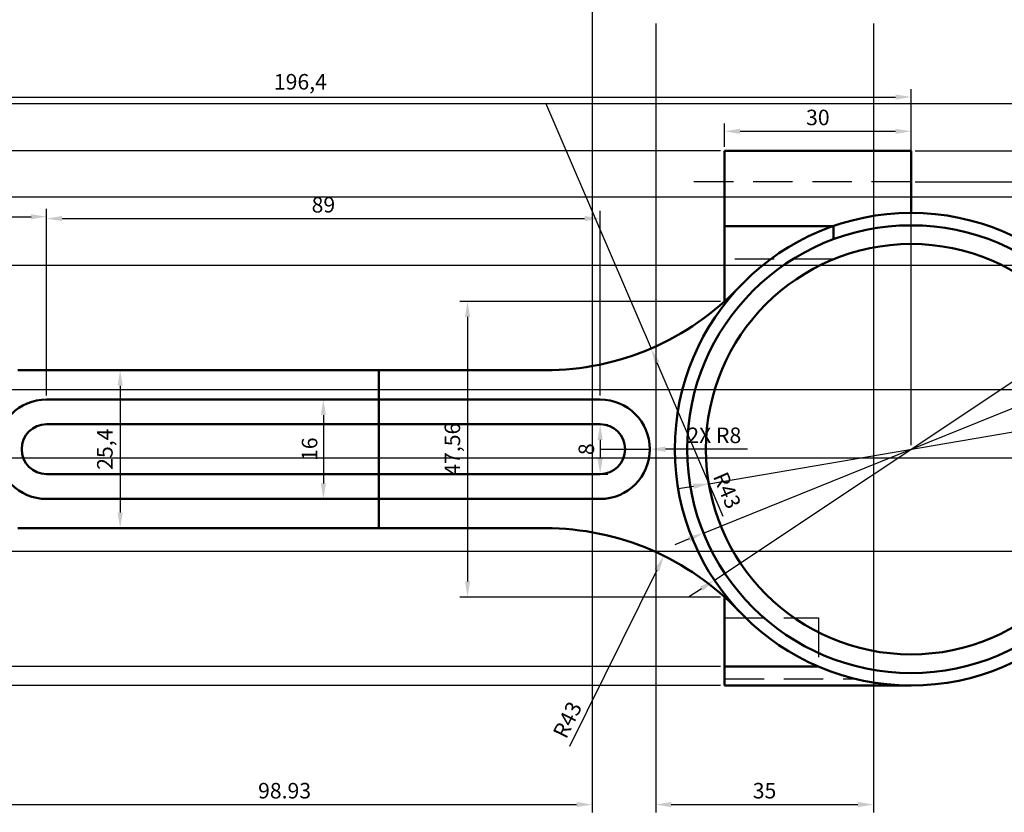
# Model space of a CAD drawing. Units: millimetres. Extents: x 1594 to 1992, y 1694 to 1927.
# Tile 2 of 4: x 1698 to 1856, y 1694 to 1822. Entities that reach past the tile are written whole.
import ezdxf

# ---------------------------------------------------------------- set-up
doc = ezdxf.new("R2010")
doc.units = ezdxf.units.MM
doc.linetypes.add('HIDDEN', pattern=[9.525, 6.35, -3.175])
for name, color, linetype, lineweight in [('M-DIMS', 2, 'Continuous', 25), ('M-HIDN', 4, 'HIDDEN', 25), ('M-OUTL', 7, 'Continuous', 50)]:
    doc.layers.add(name, color=color, linetype=linetype, lineweight=lineweight)
doc.styles.get("Standard").update_dxf_attribs({"font": 'arial.ttf'})
doc.dimstyles.new('ISO-25', dxfattribs={"dimtxt": 2.5, "dimasz": 2.5, "dimexe": 1.25, "dimexo": 0.625, "dimtad": 1, "dimtxsty": 'Standard', "dimcen": 2.5, "dimadec": 0, "dimazin": 0, "dimtfac": 1, "dimtmove": 0, "dimatfit": 3, "dimfxl": 1, "dimarcsym": 0})

# ---------------------------------------------------------------- blocks, each defined once
blk = doc.blocks.new('*D13')
at = {"layer": 'Defpoints', "color": 0, "transparency": 16777216}
for p in [(1701.91, 1789.89), (1701.91, 1760.5), (1669.71, 1752.5)]:
    blk.add_point(p, dxfattribs=at)
at = {"layer": 'M-DIMS', "color": 0, "lineweight": -2, "transparency": 16777216}
for p, q in [((1669.71, 1753.13), (1669.71, 1791.14)), ((1701.91, 1761.13), (1701.91, 1791.14)), ((1672.21, 1789.89), (1699.41, 1789.89))]:
    blk.add_line(p, q, dxfattribs=at)
at = {"layer": 'M-DIMS', "color": 0, "transparency": 16777216}
for points in [[(1672.21, 1790.3), (1672.21, 1789.47), (1669.71, 1789.89)], [(1699.41, 1790.3), (1699.41, 1789.47), (1701.91, 1789.89)]]:
    blk.add_solid(points, dxfattribs=at)
at = {"layer": 'M-DIMS', "color": 0, "transparency": 16777216, "insert": (1685.81, 1792.01), "char_height": 2.5, "attachment_point": 5}
blk.add_mtext('32,2', dxfattribs=at)
blk = doc.blocks.new('*D14')
at = {"layer": 'Defpoints', "color": 0, "transparency": 16777216}
for p in [(1790.91, 1789.59), (1701.91, 1760.5), (1790.91, 1760.5)]:
    blk.add_point(p, dxfattribs=at)
at = {"layer": 'M-DIMS', "color": 0, "lineweight": -2, "transparency": 16777216}
for p, q in [((1701.91, 1761.13), (1701.91, 1790.84)), ((1790.91, 1761.13), (1790.91, 1790.84)), ((1704.41, 1789.59), (1788.41, 1789.59))]:
    blk.add_line(p, q, dxfattribs=at)
at = {"layer": 'M-DIMS', "color": 0, "transparency": 16777216}
for points in [[(1704.41, 1790.01), (1704.41, 1789.18), (1701.91, 1789.59)], [(1788.41, 1790.01), (1788.41, 1789.18), (1790.91, 1789.59)]]:
    blk.add_solid(points, dxfattribs=at)
at = {"layer": 'M-DIMS', "color": 0, "transparency": 16777216, "insert": (1746.41, 1791.49), "char_height": 2.5, "attachment_point": 5}
blk.add_mtext('89', dxfattribs=at)
blk = doc.blocks.new('*D16')
at = {"layer": 'Defpoints', "color": 0, "transparency": 16777216}
for p in [(1840.91, 1809.14), (1644.51, 1752.5), (1840.91, 1752.5)]:
    blk.add_point(p, dxfattribs=at)
at = {"layer": 'M-DIMS', "color": 0, "lineweight": -2, "transparency": 16777216}
for p, q in [((1644.51, 1753.13), (1644.51, 1810.39)), ((1840.91, 1753.13), (1840.91, 1810.39)), ((1647.01, 1809.14), (1838.41, 1809.14))]:
    blk.add_line(p, q, dxfattribs=at)
at = {"layer": 'M-DIMS', "color": 0, "transparency": 16777216}
for points in [[(1647.01, 1809.56), (1647.01, 1808.72), (1644.51, 1809.14)], [(1838.41, 1809.56), (1838.41, 1808.72), (1840.91, 1809.14)]]:
    blk.add_solid(points, dxfattribs=at)
at = {"layer": 'M-DIMS', "color": 0, "transparency": 16777216, "insert": (1742.71, 1811.27), "char_height": 2.5, "attachment_point": 5}
blk.add_mtext('196,4', dxfattribs=at)
blk = doc.blocks.new('*D17')
at = {"layer": 'Defpoints', "color": 0, "transparency": 16777216}
for p in [(1840.91, 1803.63), (1810.91, 1800.5), (1840.91, 1800.5)]:
    blk.add_point(p, dxfattribs=at)
at = {"layer": 'M-DIMS', "color": 0, "lineweight": -2, "transparency": 16777216}
for p, q in [((1810.91, 1801.13), (1810.91, 1804.88)), ((1840.91, 1801.13), (1840.91, 1804.88)), ((1813.41, 1803.63), (1838.41, 1803.63))]:
    blk.add_line(p, q, dxfattribs=at)
at = {"layer": 'M-DIMS', "color": 0, "transparency": 16777216}
for points in [[(1813.41, 1804.04), (1813.41, 1803.21), (1810.91, 1803.63)], [(1838.41, 1804.04), (1838.41, 1803.21), (1840.91, 1803.63)]]:
    blk.add_solid(points, dxfattribs=at)
at = {"layer": 'M-DIMS', "color": 0, "transparency": 16777216, "insert": (1825.91, 1805.53), "char_height": 2.5, "attachment_point": 5}
blk.add_mtext('30', dxfattribs=at)
blk = doc.blocks.new('*D18')
at = {"layer": 'Defpoints', "color": 0, "transparency": 16777216}
for p in [(1726.28, 1765.2), (1713.73, 1739.8), (1726.28, 1739.8)]:
    blk.add_point(p, dxfattribs=at)
at = {"layer": 'M-DIMS', "color": 0, "lineweight": -2, "transparency": 16777216}
for p, q in [((1725.66, 1765.2), (1712.48, 1765.2)), ((1713.73, 1762.7), (1713.73, 1742.3)), ((1725.66, 1739.8), (1712.48, 1739.8))]:
    blk.add_line(p, q, dxfattribs=at)
at = {"layer": 'M-DIMS', "color": 0, "transparency": 16777216}
for points in [[(1713.32, 1762.7), (1714.15, 1762.7), (1713.73, 1765.2)], [(1713.32, 1742.3), (1714.15, 1742.3), (1713.73, 1739.8)]]:
    blk.add_solid(points, dxfattribs=at)
at = {"layer": 'M-DIMS', "color": 0, "transparency": 16777216, "insert": (1711.6, 1752.5), "char_height": 2.5, "attachment_point": 5, "rotation": 90}
blk.add_mtext('25,4', dxfattribs=at)
blk = doc.blocks.new('*D19')
at = {"layer": 'Defpoints', "color": 0, "transparency": 16777216}
for p in [(1746.41, 1760.5), (1746.41, 1744.5), (1746.41, 1744.5)]:
    blk.add_point(p, dxfattribs=at)
at = {"layer": 'M-DIMS', "color": 0, "lineweight": -2, "transparency": 16777216}
for p, q in [((1747.03, 1760.5), (1747.66, 1760.5)), ((1746.41, 1758), (1746.41, 1747)), ((1747.03, 1744.5), (1747.66, 1744.5))]:
    blk.add_line(p, q, dxfattribs=at)
at = {"layer": 'M-DIMS', "color": 0, "transparency": 16777216}
for points in [[(1745.99, 1758), (1746.82, 1758), (1746.41, 1760.5)], [(1745.99, 1747), (1746.82, 1747), (1746.41, 1744.5)]]:
    blk.add_solid(points, dxfattribs=at)
at = {"layer": 'M-DIMS', "color": 0, "transparency": 16777216, "insert": (1744.51, 1752.5), "char_height": 2.5, "attachment_point": 5, "rotation": 90}
blk.add_mtext('16', dxfattribs=at)
blk = doc.blocks.new('*D20')
at = {"layer": 'Defpoints', "color": 0, "transparency": 16777216}
for p in [(1746.41, 1756.5), (1746.41, 1748.5), (1790.91, 1748.5)]:
    blk.add_point(p, dxfattribs=at)
at = {"layer": 'M-DIMS', "color": 0, "lineweight": -2, "transparency": 16777216}
for p, q in [((1747.03, 1756.5), (1792.16, 1756.5)), ((1790.91, 1754), (1790.91, 1751)), ((1747.03, 1748.5), (1792.16, 1748.5))]:
    blk.add_line(p, q, dxfattribs=at)
at = {"layer": 'M-DIMS', "color": 0, "transparency": 16777216}
for points in [[(1790.49, 1754), (1791.32, 1754), (1790.91, 1756.5)], [(1790.49, 1751), (1791.32, 1751), (1790.91, 1748.5)]]:
    blk.add_solid(points, dxfattribs=at)
at = {"layer": 'M-DIMS', "color": 0, "transparency": 16777216, "insert": (1789.01, 1752.5), "char_height": 2.5, "attachment_point": 5, "rotation": 90}
blk.add_mtext('8', dxfattribs=at)
blk = doc.blocks.new('*D21')
at = {"layer": 'Defpoints', "color": 0, "transparency": 16777216}
for p in [(1810.91, 1776.28), (1769.59, 1728.73), (1810.91, 1728.73)]:
    blk.add_point(p, dxfattribs=at)
at = {"layer": 'M-DIMS', "color": 0, "lineweight": -2, "transparency": 16777216}
for p, q in [((1810.28, 1776.28), (1768.34, 1776.28)), ((1769.59, 1773.78), (1769.59, 1731.23)), ((1810.28, 1728.73), (1768.34, 1728.73))]:
    blk.add_line(p, q, dxfattribs=at)
at = {"layer": 'M-DIMS', "color": 0, "transparency": 16777216}
for points in [[(1769.18, 1773.78), (1770.01, 1773.78), (1769.59, 1776.28)], [(1769.18, 1731.23), (1770.01, 1731.23), (1769.59, 1728.73)]]:
    blk.add_solid(points, dxfattribs=at)
at = {"layer": 'M-DIMS', "color": 0, "transparency": 16777216, "insert": (1767.47, 1752.5), "char_height": 2.5, "attachment_point": 5, "rotation": 90}
blk.add_mtext('47,56', dxfattribs=at)
blk = doc.blocks.new('*D24')
at = {"layer": 'Defpoints', "color": 0, "transparency": 16777216}
for p in [(1801.16, 1735.35), (1782.1, 1696.8)]:
    blk.add_point(p, dxfattribs=at)
at = {"layer": 'M-DIMS', "color": 0, "lineweight": -2, "transparency": 16777216}
blk.add_line((1786.03, 1704.76), (1800.05, 1733.11), dxfattribs=at)
at = {"layer": 'M-DIMS', "color": 0, "transparency": 16777216}
blk.add_solid([(1799.68, 1733.29), (1800.42, 1732.92), (1801.16, 1735.35)], dxfattribs=at)
at = {"layer": 'M-DIMS', "color": 0, "transparency": 16777216, "insert": (1785.93, 1708.84), "char_height": 2.5, "attachment_point": 5, "rotation": 63.6879}
blk.add_mtext('R43', dxfattribs=at)
blk = doc.blocks.new('*D28')
at = {"layer": 'Defpoints', "color": 0, "transparency": 16777216}
for p in [(1872.54, 1773.56), (1809.27, 1731.45)]:
    blk.add_point(p, dxfattribs=at)
at = {"layer": 'M-DIMS', "color": 0, "lineweight": -2, "transparency": 16777216}
for p, q in [((1891.75, 1786.34), (1874.62, 1774.94)), ((1809.27, 1731.45), (1872.54, 1773.56)), ((1807.19, 1730.07), (1805.11, 1728.68))]:
    blk.add_line(p, q, dxfattribs=at)
at = {"layer": 'M-DIMS', "color": 0, "transparency": 16777216}
for points in [[(1874.39, 1775.29), (1874.85, 1774.59), (1872.54, 1773.56)], [(1806.96, 1730.42), (1807.42, 1729.72), (1809.27, 1731.45)]]:
    blk.add_solid(points, dxfattribs=at)
at = {"layer": 'M-DIMS', "color": 0, "transparency": 16777216, "insert": (1887.51, 1785.89), "char_height": 2.5, "attachment_point": 5, "rotation": 33.6408}
blk.add_mtext('∅76', dxfattribs=at)
blk = doc.blocks.new('*D29')
at = {"layer": 'Defpoints', "color": 0, "transparency": 16777216}
for p in [(1874.28, 1766), (1807.53, 1739.01)]:
    blk.add_point(p, dxfattribs=at)
at = {"layer": 'M-DIMS', "color": 0, "lineweight": -2, "transparency": 16777216}
for p, q in [((1897.51, 1775.4), (1876.6, 1766.94)), ((1807.53, 1739.01), (1874.28, 1766)), ((1805.22, 1738.07), (1802.9, 1737.13))]:
    blk.add_line(p, q, dxfattribs=at)
at = {"layer": 'M-DIMS', "color": 0, "transparency": 16777216}
for points in [[(1876.44, 1767.33), (1876.75, 1766.55), (1874.28, 1766)], [(1805.06, 1738.46), (1805.37, 1737.68), (1807.53, 1739.01)]]:
    blk.add_solid(points, dxfattribs=at)
at = {"layer": 'M-DIMS', "color": 0, "transparency": 16777216, "insert": (1893.28, 1775.81), "char_height": 2.5, "attachment_point": 5, "rotation": 22.0218}
blk.add_mtext('∅72', dxfattribs=at)
blk = doc.blocks.new('*D30')
at = {"layer": 'Defpoints', "color": 0, "transparency": 16777216}
for p in [(1873.44, 1758.06), (1808.38, 1746.95)]:
    blk.add_point(p, dxfattribs=at)
at = {"layer": 'M-DIMS', "color": 0, "lineweight": -2, "transparency": 16777216}
for p, q in [((1899.42, 1762.5), (1875.9, 1758.48)), ((1808.38, 1746.95), (1873.44, 1758.06)), ((1805.91, 1746.53), (1803.45, 1746.11))]:
    blk.add_line(p, q, dxfattribs=at)
at = {"layer": 'M-DIMS', "color": 0, "transparency": 16777216}
for points in [[(1875.83, 1758.89), (1875.97, 1758.07), (1873.44, 1758.06)], [(1805.84, 1746.94), (1805.98, 1746.12), (1808.38, 1746.95)]]:
    blk.add_solid(points, dxfattribs=at)
at = {"layer": 'M-DIMS', "color": 0, "transparency": 16777216, "insert": (1895.37, 1763.81), "char_height": 2.5, "attachment_point": 5, "rotation": 9.6936}
blk.add_mtext('∅66', dxfattribs=at)
blk = doc.blocks.new('*D39')
at = {"layer": 'Defpoints', "color": 0, "transparency": 16777216}
for p in [(1840.91, 1800.5), (1840.91, 1795.5), (1985.18, 1795.5)]:
    blk.add_point(p, dxfattribs=at)
at = {"layer": 'M-DIMS', "color": 0, "lineweight": -2, "transparency": 16777216}
for p, q in [((1985.18, 1803), (1985.18, 1805.5)), ((1841.53, 1800.5), (1986.43, 1800.5)), ((1985.18, 1800.5), (1985.18, 1795.5)), ((1841.53, 1795.5), (1986.43, 1795.5)), ((1985.18, 1793), (1985.18, 1790.5))]:
    blk.add_line(p, q, dxfattribs=at)
at = {"layer": 'M-DIMS', "color": 0, "transparency": 16777216}
for points in [[(1984.76, 1803), (1985.6, 1803), (1985.18, 1800.5)], [(1984.76, 1793), (1985.6, 1793), (1985.18, 1795.5)]]:
    blk.add_solid(points, dxfattribs=at)
at = {"layer": 'M-DIMS', "color": 0, "transparency": 16777216, "insert": (1983.28, 1798), "char_height": 2.5, "attachment_point": 5, "rotation": 90}
blk.add_mtext('5', dxfattribs=at)
blk = doc.blocks.new('*D40')
at = {"layer": 'Defpoints', "color": 0, "transparency": 16777216}
for p in [(1810.91, 1800.5), (1597.57, 1714.5), (1810.91, 1714.5)]:
    blk.add_point(p, dxfattribs=at)
at = {"layer": 'M-DIMS', "color": 0, "lineweight": -2, "transparency": 16777216}
for p, q in [((1810.28, 1800.5), (1596.32, 1800.5)), ((1597.57, 1798), (1597.57, 1717)), ((1810.28, 1714.5), (1596.32, 1714.5))]:
    blk.add_line(p, q, dxfattribs=at)
at = {"layer": 'M-DIMS', "color": 0, "transparency": 16777216}
for points in [[(1597.15, 1798), (1597.99, 1798), (1597.57, 1800.5)], [(1597.15, 1717), (1597.99, 1717), (1597.57, 1714.5)]]:
    blk.add_solid(points, dxfattribs=at)
at = {"layer": 'M-DIMS', "color": 0, "transparency": 16777216, "insert": (1595.67, 1757.5), "char_height": 2.5, "attachment_point": 5, "rotation": 90}
blk.add_mtext('86', dxfattribs=at)
blk = doc.blocks.new('*D41')
at = {"layer": 'Defpoints', "color": 0, "transparency": 16777216}
for p in [(1810.91, 1717.55), (1597.57, 1714.5), (1810.91, 1714.5)]:
    blk.add_point(p, dxfattribs=at)
at = {"layer": 'M-DIMS', "color": 0, "lineweight": -2, "transparency": 16777216}
for p, q in [((1597.57, 1720.05), (1597.57, 1722.55)), ((1810.28, 1717.55), (1596.32, 1717.55)), ((1597.57, 1717.55), (1597.57, 1714.5)), ((1810.28, 1714.5), (1596.32, 1714.5)), ((1597.57, 1712), (1597.57, 1701.74))]:
    blk.add_line(p, q, dxfattribs=at)
at = {"layer": 'M-DIMS', "color": 0, "transparency": 16777216}
for points in [[(1597.15, 1720.05), (1597.99, 1720.05), (1597.57, 1717.55)], [(1597.15, 1712), (1597.99, 1712), (1597.57, 1714.5)]]:
    blk.add_solid(points, dxfattribs=at)
at = {"layer": 'M-DIMS', "color": 0, "transparency": 16777216, "insert": (1595.67, 1705.62), "char_height": 2.5, "attachment_point": 5, "rotation": 90}
blk.add_mtext('3.05', dxfattribs=at)
blk = doc.blocks.new('*D44')
at = {"layer": 'Defpoints', "color": 0, "transparency": 16777216}
for p in [(1932.03, 1782.06), (1597.57, 1762.06), (1932.03, 1762.06)]:
    blk.add_point(p, dxfattribs=at)
at = {"layer": 'M-DIMS', "color": 0, "lineweight": -2, "transparency": 16777216}
for p, q in [((1931.4, 1782.06), (1596.32, 1782.06)), ((1597.57, 1779.56), (1597.57, 1764.56)), ((1931.4, 1762.06), (1596.32, 1762.06))]:
    blk.add_line(p, q, dxfattribs=at)
at = {"layer": 'M-DIMS', "color": 0, "transparency": 16777216}
for points in [[(1597.15, 1779.56), (1597.99, 1779.56), (1597.57, 1782.06)], [(1597.15, 1764.56), (1597.99, 1764.56), (1597.57, 1762.06)]]:
    blk.add_solid(points, dxfattribs=at)
at = {"layer": 'M-DIMS', "color": 0, "transparency": 16777216, "insert": (1595.67, 1772.06), "char_height": 2.5, "attachment_point": 5, "rotation": 90}
blk.add_mtext('20', dxfattribs=at)
blk = doc.blocks.new('*D45')
at = {"layer": 'Defpoints', "color": 0, "transparency": 16777216}
for p in [(1922.03, 1808.06), (1597.57, 1793.06), (1922.03, 1793.06)]:
    blk.add_point(p, dxfattribs=at)
at = {"layer": 'M-DIMS', "color": 0, "lineweight": -2, "transparency": 16777216}
for p, q in [((1921.4, 1808.06), (1596.32, 1808.06)), ((1597.57, 1805.56), (1597.57, 1795.56)), ((1921.4, 1793.06), (1596.32, 1793.06))]:
    blk.add_line(p, q, dxfattribs=at)
at = {"layer": 'M-DIMS', "color": 0, "transparency": 16777216}
for points in [[(1597.15, 1805.56), (1597.99, 1805.56), (1597.57, 1808.06)], [(1597.15, 1795.56), (1597.99, 1795.56), (1597.57, 1793.06)]]:
    blk.add_solid(points, dxfattribs=at)
at = {"layer": 'M-DIMS', "color": 0, "transparency": 16777216, "insert": (1595.67, 1800.56), "char_height": 2.5, "attachment_point": 5, "rotation": 90}
blk.add_mtext('15', dxfattribs=at)
blk = doc.blocks.new('*D46')
at = {"layer": 'Defpoints', "color": 0, "transparency": 16777216}
for p in [(1922.03, 1751.06), (1597.57, 1736.06), (1922.03, 1736.06)]:
    blk.add_point(p, dxfattribs=at)
at = {"layer": 'M-DIMS', "color": 0, "lineweight": -2, "transparency": 16777216}
for p, q in [((1921.4, 1751.06), (1596.32, 1751.06)), ((1597.57, 1748.56), (1597.57, 1738.56)), ((1921.4, 1736.06), (1596.32, 1736.06))]:
    blk.add_line(p, q, dxfattribs=at)
at = {"layer": 'M-DIMS', "color": 0, "transparency": 16777216}
for points in [[(1597.15, 1748.56), (1597.99, 1748.56), (1597.57, 1751.06)], [(1597.15, 1738.56), (1597.99, 1738.56), (1597.57, 1736.06)]]:
    blk.add_solid(points, dxfattribs=at)
at = {"layer": 'M-DIMS', "color": 0, "transparency": 16777216, "insert": (1595.67, 1743.56), "char_height": 2.5, "attachment_point": 5, "rotation": 90}
blk.add_mtext('15', dxfattribs=at)
blk = doc.blocks.new('*D50')
at = {"layer": 'Defpoints', "color": 0, "transparency": 16777216}
for p in [(1690.7, 1831.92), (1789.63, 1831.92), (1789.63, 1695.35)]:
    blk.add_point(p, dxfattribs=at)
at = {"layer": 'M-DIMS', "color": 0, "lineweight": -2, "transparency": 16777216}
for p, q in [((1690.7, 1831.3), (1690.7, 1694.1)), ((1789.63, 1831.3), (1789.63, 1694.1)), ((1693.2, 1695.35), (1787.13, 1695.35))]:
    blk.add_line(p, q, dxfattribs=at)
at = {"layer": 'M-DIMS', "color": 0, "transparency": 16777216}
for points in [[(1693.2, 1695.77), (1693.2, 1694.94), (1690.7, 1695.35)], [(1787.13, 1695.77), (1787.13, 1694.94), (1789.63, 1695.35)]]:
    blk.add_solid(points, dxfattribs=at)
at = {"layer": 'M-DIMS', "color": 0, "transparency": 16777216, "insert": (1740.17, 1697.26), "char_height": 2.5, "attachment_point": 5}
blk.add_mtext('98.93', dxfattribs=at)
blk = doc.blocks.new('*D51')
at = {"layer": 'Defpoints', "color": 0, "transparency": 16777216}
for p in [(1799.84, 1821.58), (1834.84, 1821.58), (1834.84, 1695.35)]:
    blk.add_point(p, dxfattribs=at)
at = {"layer": 'M-DIMS', "color": 0, "lineweight": -2, "transparency": 16777216}
for p, q in [((1799.84, 1820.95), (1799.84, 1694.1)), ((1834.84, 1820.95), (1834.84, 1694.1)), ((1802.34, 1695.35), (1832.34, 1695.35))]:
    blk.add_line(p, q, dxfattribs=at)
at = {"layer": 'M-DIMS', "color": 0, "transparency": 16777216}
for points in [[(1802.34, 1695.77), (1802.34, 1694.94), (1799.84, 1695.35)], [(1832.34, 1695.77), (1832.34, 1694.94), (1834.84, 1695.35)]]:
    blk.add_solid(points, dxfattribs=at)
at = {"layer": 'M-DIMS', "color": 0, "transparency": 16777216, "insert": (1817.34, 1697.26), "char_height": 2.5, "attachment_point": 5}
blk.add_mtext('35', dxfattribs=at)
blk = doc.blocks.new('*D59')
at = {"layer": 'Defpoints', "color": 0, "transparency": 16777216}
for p in [(1782.1, 1808.2), (1799.09, 1768.71)]:
    blk.add_point(p, dxfattribs=at)
at = {"layer": 'M-DIMS', "color": 0, "lineweight": -2, "transparency": 16777216}
for p, q in [((1782.1, 1808.2), (1799.09, 1768.71)), ((1810.71, 1741.69), (1800.08, 1766.41))]:
    blk.add_line(p, q, dxfattribs=at)
at = {"layer": 'M-DIMS', "color": 0, "transparency": 16777216}
blk.add_solid([(1800.46, 1766.57), (1799.7, 1766.24), (1799.09, 1768.71)], dxfattribs=at)
at = {"layer": 'M-DIMS', "color": 0, "transparency": 16777216, "insert": (1811.03, 1745.76), "char_height": 2.5, "attachment_point": 5, "rotation": 293.2779}
blk.add_mtext('R43', dxfattribs=at)
blk = doc.blocks.new('*D60')
at = {"layer": 'Defpoints', "color": 0, "transparency": 16777216}
for p in [(1790.91, 1752.5), (1798.91, 1752.51)]:
    blk.add_point(p, dxfattribs=at)
at = {"layer": 'M-DIMS', "color": 0, "lineweight": -2, "transparency": 16777216}
for p, q in [((1790.91, 1752.5), (1798.91, 1752.51)), ((1814.61, 1752.51), (1801.41, 1752.51))]:
    blk.add_line(p, q, dxfattribs=at)
at = {"layer": 'M-DIMS', "color": 0, "transparency": 16777216}
blk.add_solid([(1801.41, 1752.92), (1801.41, 1752.09), (1798.91, 1752.51)], dxfattribs=at)
at = {"layer": 'M-DIMS', "color": 0, "transparency": 16777216, "insert": (1809.26, 1754.41), "char_height": 2.5, "attachment_point": 5, "rotation": 0.0015}
blk.add_mtext('2X R8', dxfattribs=at)

msp = doc.modelspace()

# ---------------------------------------------------------------- linework, layer by layer
at = {"layer": 'M-HIDN'}
for p, q in [((1840.9068, 1795.5048), (1803.2857, 1795.5048)), ((1828.4172, 1783.05), (1810.9068, 1783.05)), ((1810.9068, 1725.4011), (1825.9908, 1725.4011)), ((1825.9908, 1725.4011), (1825.9908, 1717.5546)), ((1810.9068, 1715.5546), (1832.0363, 1715.5546))]:
    msp.add_line(p, q, dxfattribs=at)
at = {"layer": 'M-OUTL'}
for p, q in [((1840.9068, 1800.5048), (1810.9068, 1800.5048)), ((1810.9068, 1800.5048), (1810.9068, 1776.2824)), ((1840.9068, 1790.5048), (1840.9068, 1800.5048)), ((1810.9068, 1788.3936), (1828.4172, 1788.3936)), ((1828.4172, 1788.3936), (1828.4172, 1786.2688)), ((1755.3068, 1765.2048), (1697.2577, 1765.2048)), ((1755.3068, 1752.5048), (1755.3068, 1765.2048)), ((1755.3068, 1765.2048), (1782.0977, 1765.2048)), ((1701.9068, 1760.5048), (1790.9068, 1760.5048)), ((1701.9068, 1756.5048), (1790.9068, 1756.5048)), ((1755.3068, 1752.5048), (1755.3068, 1739.8048)), ((1790.9068, 1748.5048), (1701.9068, 1748.5048)), ((1790.9068, 1744.5048), (1701.9068, 1744.5048)), ((1755.3068, 1739.8048), (1697.2577, 1739.8048)), ((1755.3068, 1739.8048), (1782.0977, 1739.8048)), ((1810.9068, 1728.7271), (1810.9068, 1714.5048)), ((1825.9908, 1717.5546), (1810.9068, 1717.5546)), ((1840.9068, 1714.5048), (1810.9068, 1714.5048))]:
    msp.add_line(p, q, dxfattribs=at)
for radius in [38, 36, 33]:
    msp.add_circle((1840.9068, 1752.5048), radius, dxfattribs=at)
for centre, radius, start, end in [((1782.0977, 1808.2048), 43, 270, 316.555286), ((1701.9068, 1752.5048), 8, 90, 270), ((1790.9068, 1752.5048), 8, 270, 90), ((1701.9068, 1752.5048), 4, 90, 270), ((1790.9068, 1752.5048), 4, 270, 90), ((1782.0977, 1696.8048), 43, 43.444714, 90)]:
    msp.add_arc(centre, radius, start, end, dxfattribs=at)

# ---------------------------------------------------------------- dimensions: what is measured, and where the dimension line sits
at = {"layer": 'M-DIMS'}
for base, p1, p2, override, picture, middle in [((1789.6319, 1695.3548), (1690.7029, 1831.9212), (1789.6319, 1831.9212), {"dimdec": 2, "dimlfac": 1, "dimrnd": 0, "dimzin": 0, "dimdsep": 46, "dimlunit": 2}, '*D50', (1740.1674, 1697.2571)), ((1834.8392, 1695.3548), (1799.8392, 1821.5797), (1834.8392, 1821.5797), {"dimdec": 0, "dimlfac": 1, "dimrnd": 0, "dimzin": 0, "dimdsep": 46, "dimlunit": 2}, '*D51', (1817.3392, 1697.2571)), ((1840.9068, 1809.14), (1644.5068, 1752.5048), (1840.9068, 1752.5048), {"dimclrd": 0, "dimclre": 0, "dimclrt": 0}, '*D16', (1742.7068, 1811.2674)), ((1840.9068, 1803.6273), (1810.9068, 1800.5048), (1840.9068, 1800.5048), {"dimclrd": 0, "dimclre": 0, "dimclrt": 0}, '*D17', (1825.9068, 1805.5296)), ((1701.9068, 1789.8851), (1669.7068, 1752.5048), (1701.9068, 1760.5048), {"dimclrd": 0, "dimclre": 0, "dimclrt": 0}, '*D13', (1685.8068, 1792.0125)), ((1790.9068, 1789.5934), (1701.9068, 1760.5048), (1790.9068, 1760.5048), {"dimclrd": 0, "dimclre": 0, "dimclrt": 0}, '*D14', (1746.4068, 1791.4948))]:
    dim = msp.add_linear_dim(base=base, p1=p1, p2=p2, dimstyle='ISO-25', override=override, dxfattribs=at)
    dim.commit()
    dim.dimension.update_dxf_attribs({"geometry": picture, "text_midpoint": middle})
for base, p1, p2, override, picture, middle in [((1597.571, 1793.0568), (1922.03, 1808.0568), (1922.03, 1793.0568), {"dimdec": 0, "dimlfac": 1, "dimrnd": 0, "dimzin": 0, "dimdsep": 46, "dimlunit": 2}, '*D45', (1595.6695, 1800.5568)), ((1985.18, 1795.5048), (1840.9068, 1800.5048), (1840.9068, 1795.5048), {"dimdec": 0, "dimlfac": 1, "dimrnd": 0, "dimzin": 0, "dimdsep": 46, "dimlunit": 2}, '*D39', (1983.2836, 1798.0048)), ((1597.571, 1714.5048), (1810.9068, 1800.5048), (1810.9068, 1714.5048), {"dimdec": 0, "dimlfac": 1, "dimrnd": 0, "dimzin": 0, "dimdsep": 46, "dimlunit": 2}, '*D40', (1595.6695, 1757.5048)), ((1597.571, 1762.0568), (1932.03, 1782.0568), (1932.03, 1762.0568), {"dimdec": 0, "dimlfac": 1, "dimrnd": 0, "dimzin": 0, "dimdsep": 46, "dimlunit": 2}, '*D44', (1595.6695, 1772.0568)), ((1769.5943, 1728.7271), (1810.9068, 1776.2824), (1810.9068, 1728.7271), {"dimclrd": 0, "dimclre": 0, "dimclrt": 0}, '*D21', (1767.4669, 1752.5048)), ((1713.7319, 1739.8048), (1726.2823, 1765.2048), (1726.2823, 1739.8048), {"dimclrd": 0, "dimclre": 0, "dimclrt": 0}, '*D18', (1711.6046, 1752.5048)), ((1746.4068, 1744.5048), (1746.4068, 1760.5048), (1746.4068, 1744.5048), {"dimclrd": 0, "dimclre": 0, "dimclrt": 0}, '*D19', (1744.5054, 1752.5048)), ((1790.9068, 1748.5048), (1746.4068, 1756.5048), (1746.4068, 1748.5048), {"dimclrd": 0, "dimclre": 0, "dimclrt": 0}, '*D20', (1789.0054, 1752.5048)), ((1597.571, 1736.0568), (1922.03, 1751.0568), (1922.03, 1736.0568), {"dimdec": 0, "dimlfac": 1, "dimrnd": 0, "dimzin": 0, "dimdsep": 46, "dimlunit": 2}, '*D46', (1595.6695, 1743.5568)), ((1597.571, 1714.5048), (1810.9068, 1717.5546), (1810.9068, 1714.5048), {"dimdec": 2, "dimlfac": 1, "dimrnd": 0, "dimzin": 0, "dimdsep": 46, "dimlunit": 2}, '*D41', (1595.6687, 1705.6243))]:
    dim = msp.add_linear_dim(base=base, p1=p1, p2=p2, angle=90, dimstyle='ISO-25', override=override, dxfattribs=at)
    dim.commit()
    dim.dimension.update_dxf_attribs({"geometry": picture, "text_midpoint": middle})
for center, mpoint, override, picture, middle in [((1782.0977, 1808.2048), (1799.091, 1768.705), {"dimdec": 0, "dimlfac": 1, "dimrnd": 0, "dimzin": 0, "dimdsep": 46, "dimlunit": 2}, '*D59', (1809.2869, 1745.0052)), ((1782.0977, 1696.8048), (1801.1579, 1735.3497), {"dimclrd": 0, "dimclre": 0, "dimclrt": 0}, '*D24', (1787.6324, 1707.9973))]:
    dim = msp.add_radius_dim(center=center, mpoint=mpoint, dimstyle='ISO-25', override=override, dxfattribs=at)
    dim.commit()
    dim.dimension.update_dxf_attribs({"geometry": picture, "text_midpoint": middle, "dimtype": 164})
for p1, p2, picture, middle in [((1809.2708, 1731.4534), (1872.5428, 1773.5562), '*D28', (1888.6064, 1784.2453)), ((1807.5334, 1739.0062), (1874.2803, 1766.0034), '*D29', (1894.0198, 1773.9874)), ((1808.378, 1746.9483), (1873.4357, 1758.0613), '*D30', (1895.6999, 1761.8644))]:
    dim = msp.add_diameter_dim_2p(p1=p1, p2=p2, dimstyle='ISO-25', override={"dimclrd": 0, "dimclre": 0, "dimclrt": 0}, dxfattribs=at)
    dim.commit()
    dim.dimension.update_dxf_attribs({"geometry": picture, "text_midpoint": middle, "dimtype": 163})
dim = msp.add_radius_dim(center=(1790.9068, 1752.5048), mpoint=(1798.9068, 1752.505), text='2X <>', dimstyle='ISO-25', override={"dimdec": 0, "dimlfac": 1, "dimrnd": 0, "dimzin": 0, "dimdsep": 46, "dimlunit": 2}, dxfattribs=at)
dim.commit()
dim.dimension.update_dxf_attribs({"geometry": '*D60', "text_midpoint": (1809.2572, 1754.4067)})

doc.saveas('drawing.dxf')
